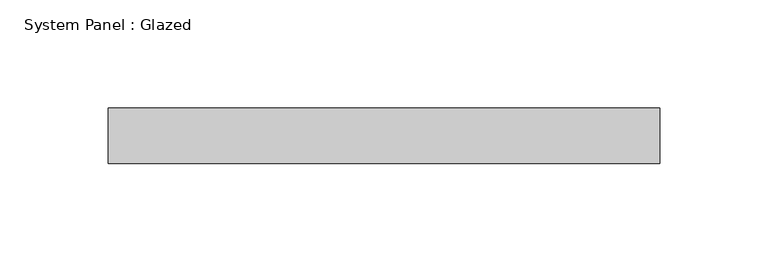
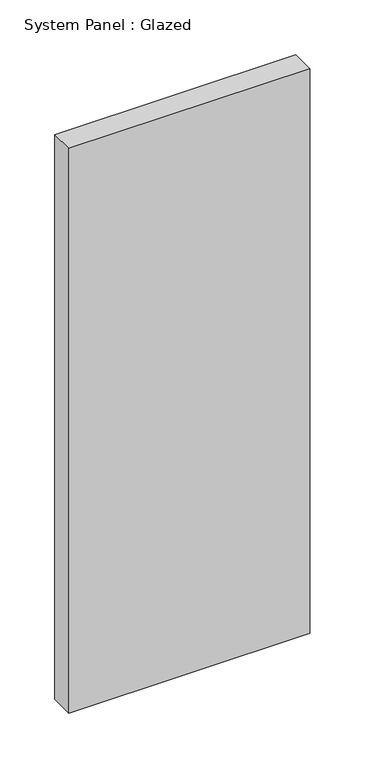
"""IFC4 building model written with IfcOpenShell, lengths in millimetres: plate geometry, System Panel : Glazed."""

from ifc_helpers import new_model, si_unit, origin, origin_with_axes, place, context, project, spatial, polyline, outline, extrude, source, transform, mapped, element, save


def system_panel_glazed_b0e64c9e(model_context):
    return source(origin(), model_context, "Body", "SweptSolid", [
        extrude(outline(polyline([(127.0, 19.05), (-127.0, 19.05), (-127.0, 44.45), (127.0, 44.45), (127.0, 19.05)])), origin_with_axes(), (0.0, 0.0, 1.0), 628.9357555),
    ])


if __name__ == "__main__":
    model = new_model("IFC4")
    model_context = context("Model", 3, world=origin())
    ifc_project = project(units=[si_unit("LENGTHUNIT", "METRE", prefix="MILLI")], contexts=[model_context])
    site = spatial("IfcSite", under=ifc_project)
    building = spatial("IfcBuilding", under=site)
    placement = place(None, origin())
    system_panel_glazed_shape = system_panel_glazed_b0e64c9e(model_context)
    element("IfcPlate", 1, ObjectType="System Panel : Glazed", at=placement, inside=building, context=model_context, shape_type="MappedRepresentation", body=[
        mapped(system_panel_glazed_shape, transform((0.0, 0.0, 0.0), x_axis=(1.0, 0.0, 0.0), y_axis=(0.0, 1.0, 0.0), z_axis=(0.0, 0.0, 1.0))),
    ])
    save(model, "model.ifc")

# Revit data of these elements
# Type "System Panel : Glazed"
#   Construction Type Id = "GSP4R"
#   Analytic Construction = "1/8 in Pilkington single glazing"
#   Visual Light Transmittance = 0.9
#   Solar Heat Gain Coefficient = 0.86
#   Heat Transfer Coefficient (U) = 1.18115 BTU/(h·ft²·°F)
#   Define Thermal Properties by = 1
# Element 1 (IfcPlate, "System Panel : Glazed")
#   Materials on its faces: "Glass"
# Materials
#   "Glass": class "Glass", colour RGB 0 128 192, transparency 0.75, Description = "Soda Lime Glass", Cost = 0
